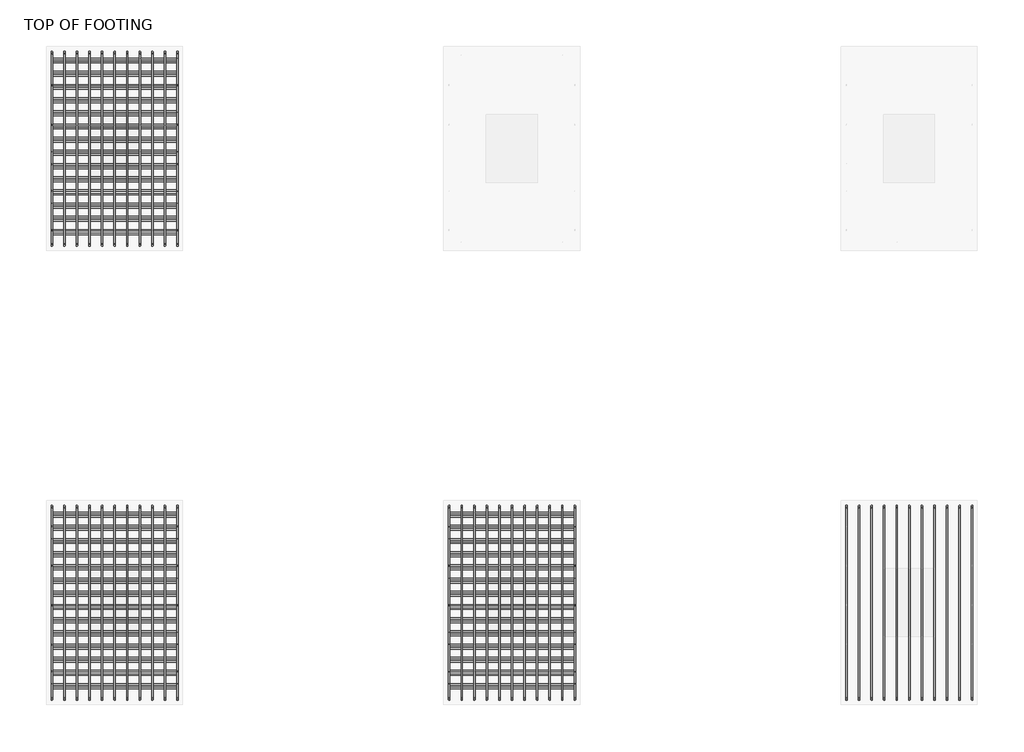
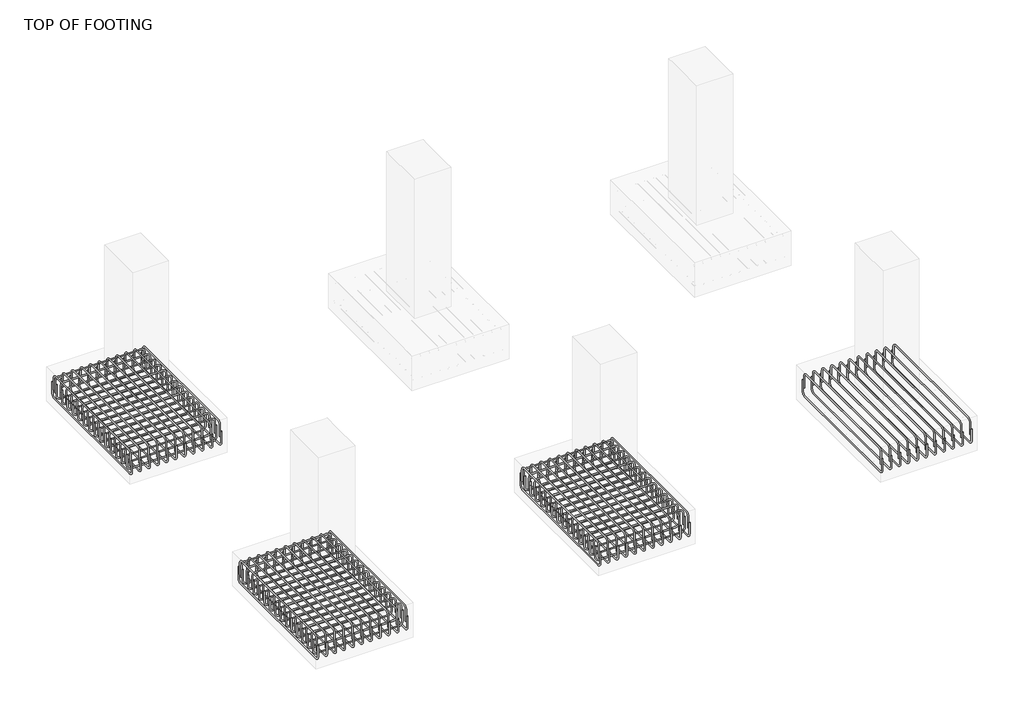
# One storey, part 3 of 11: 14 reinforcing bars.
"""IFC4 building model written with IfcOpenShell, lengths in millimetres."""

from ifc_helpers import new_model, si_unit, point, frame, origin, place, context, project, spatial, polyline, circle_curve, trimmed, segment, composite_curve, source, transform, mapped, element, save
from ifc_brep_helpers import swept_disk

model = new_model("IFC4")

# Units and contexts
model_context = context("Model", 3, world=origin())
ifc_project = project(units=[si_unit("LENGTHUNIT", "METRE", prefix="MILLI")], contexts=[model_context])

# Site, building, storey
site = spatial("IfcSite", under=ifc_project)
building = spatial("IfcBuilding", under=site)
storey = spatial("IfcBuildingStorey", under=building, Name="TOP OF FOOTING", Elevation=-1828.8)

# Reinforcing bars
placement = place(None, origin())
reinforcing_bar_shape = source(origin(), model_context, "Body", "SolidModel", [
    swept_disk(composite_curve([segment(polyline([(-8816.2384094, 6549.4712443, -2012.1658531), (-8816.2384094, 6549.4712443, -2159.4658531)]), True, "CONTINUOUS"), segment(trimmed(circle_curve(frame((-8816.2384094, 6595.8212443, -2159.4658531), z_axis=(1.0, 0.0, 0.0), x_axis=(0.0, -46.350000000000364, 0.0)), 46.35), [point((-8816.2384094, 6549.4712443, -2159.4658531))], [point((-8816.2384094, 6595.8212443, -2205.8158531))], True, "CARTESIAN"), True, "CONTINUOUS"), segment(polyline([(-8816.2384094, 6595.8212443, -2205.8158531), (-8816.2384094, 8210.4212443, -2205.8158531)]), True, "CONTINUOUS"), segment(trimmed(circle_curve(frame((-8816.2384094, 8210.4212443, -2159.4658531), z_axis=(1.0, 0.0, 0.0), x_axis=(0.0, 0.0, -46.34999999999991)), 46.35), [point((-8816.2384094, 8210.4212443, -2205.8158531))], [point((-8816.2384094, 8256.7712443, -2159.4658531))], True, "CARTESIAN"), True, "CONTINUOUS"), segment(polyline([(-8816.2384094, 8256.7712443, -2159.4658531), (-8816.2384094, 8256.7712443, -2012.1658531)]), True, "CONTINUOUS")], self_intersect=False), 6.35),
])
element("IfcReinforcingBar", 1, at=placement, inside=storey, context=model_context, shape_type="MappedRepresentation", body=[
    mapped(reinforcing_bar_shape, transform((0.0, 0.0, 0.0), x_axis=(1.0, 0.0, 0.0), y_axis=(0.0, 1.0, 0.0), z_axis=(0.0, 0.0, 1.0))),
    mapped(reinforcing_bar_shape, transform((-110.73, 0.0, 0.0), x_axis=(1.0, 0.0, 0.0), y_axis=(0.0, 1.0, 0.0), z_axis=(0.0, 0.0, 1.0))),
    mapped(reinforcing_bar_shape, transform((-221.46, 0.0, 0.0), x_axis=(1.0, 0.0, 0.0), y_axis=(0.0, 1.0, 0.0), z_axis=(0.0, 0.0, 1.0))),
    mapped(reinforcing_bar_shape, transform((-332.19, 0.0, 0.0), x_axis=(1.0, 0.0, 0.0), y_axis=(0.0, 1.0, 0.0), z_axis=(0.0, 0.0, 1.0))),
    mapped(reinforcing_bar_shape, transform((-442.92, 0.0, 0.0), x_axis=(1.0, 0.0, 0.0), y_axis=(0.0, 1.0, 0.0), z_axis=(0.0, 0.0, 1.0))),
    mapped(reinforcing_bar_shape, transform((-553.65, 0.0, 0.0), x_axis=(1.0, 0.0, 0.0), y_axis=(0.0, 1.0, 0.0), z_axis=(0.0, 0.0, 1.0))),
    mapped(reinforcing_bar_shape, transform((-664.38, 0.0, 0.0), x_axis=(1.0, 0.0, 0.0), y_axis=(0.0, 1.0, 0.0), z_axis=(0.0, 0.0, 1.0))),
    mapped(reinforcing_bar_shape, transform((-775.11, 0.0, 0.0), x_axis=(1.0, 0.0, 0.0), y_axis=(0.0, 1.0, 0.0), z_axis=(0.0, 0.0, 1.0))),
    mapped(reinforcing_bar_shape, transform((-885.84, 0.0, 0.0), x_axis=(1.0, 0.0, 0.0), y_axis=(0.0, 1.0, 0.0), z_axis=(0.0, 0.0, 1.0))),
    mapped(reinforcing_bar_shape, transform((-996.57, 0.0, 0.0), x_axis=(1.0, 0.0, 0.0), y_axis=(0.0, 1.0, 0.0), z_axis=(0.0, 0.0, 1.0))),
    mapped(reinforcing_bar_shape, transform((-1107.3, 0.0, 0.0), x_axis=(1.0, 0.0, 0.0), y_axis=(0.0, 1.0, 0.0), z_axis=(0.0, 0.0, 1.0))),
])
reinforcing_bar_2_shape = source(origin(), model_context, "Body", "SolidModel", [
    swept_disk(composite_curve([segment(polyline([(-9923.5384094, 6577.6603603, -2096.8914539), (-9923.5384094, 6577.6603603, -1949.5914539)]), True, "CONTINUOUS"), segment(trimmed(circle_curve(frame((-9923.5384094, 6624.0103603, -1949.5914539), z_axis=(-1.0, 0.0, 0.0), x_axis=(0.0, -46.349999999999454, 0.0)), 46.35), [point((-9923.5384094, 6577.6603603, -1949.5914539))], [point((-9923.5384094, 6624.0103603, -1903.2414539))], True, "CARTESIAN"), True, "CONTINUOUS"), segment(polyline([(-9923.5384094, 6624.0103603, -1903.2414539), (-9923.5384094, 8181.3238837, -1903.2414539)]), True, "CONTINUOUS"), segment(trimmed(circle_curve(frame((-9923.5384094, 8181.3238837, -1949.5914539), z_axis=(-1.0, 0.0, 0.0), x_axis=(0.0, 0.0, 46.350000000000136)), 46.35), [point((-9923.5384094, 8181.3238837, -1903.2414539))], [point((-9923.5384094, 8227.6738837, -1949.5914539))], True, "CARTESIAN"), True, "CONTINUOUS"), segment(polyline([(-9923.5384094, 8227.6738837, -1949.5914539), (-9923.5384094, 8227.6738837, -2096.8914539)]), True, "CONTINUOUS")], self_intersect=False), 6.35),
])
element("IfcReinforcingBar", 2, at=placement, inside=storey, context=model_context, shape_type="MappedRepresentation", body=[
    mapped(reinforcing_bar_2_shape, transform((0.0, 0.0, 0.0), x_axis=(1.0, 0.0, 0.0), y_axis=(0.0, 1.0, 0.0), z_axis=(0.0, 0.0, 1.0))),
    mapped(reinforcing_bar_2_shape, transform((110.73, 0.0, 0.0), x_axis=(1.0, 0.0, 0.0), y_axis=(0.0, 1.0, 0.0), z_axis=(0.0, 0.0, 1.0))),
    mapped(reinforcing_bar_2_shape, transform((221.46, 0.0, 0.0), x_axis=(1.0, 0.0, 0.0), y_axis=(0.0, 1.0, 0.0), z_axis=(0.0, 0.0, 1.0))),
    mapped(reinforcing_bar_2_shape, transform((332.19, 0.0, 0.0), x_axis=(1.0, 0.0, 0.0), y_axis=(0.0, 1.0, 0.0), z_axis=(0.0, 0.0, 1.0))),
    mapped(reinforcing_bar_2_shape, transform((442.92, 0.0, 0.0), x_axis=(1.0, 0.0, 0.0), y_axis=(0.0, 1.0, 0.0), z_axis=(0.0, 0.0, 1.0))),
    mapped(reinforcing_bar_2_shape, transform((553.65, 0.0, 0.0), x_axis=(1.0, 0.0, 0.0), y_axis=(0.0, 1.0, 0.0), z_axis=(0.0, 0.0, 1.0))),
    mapped(reinforcing_bar_2_shape, transform((664.38, 0.0, 0.0), x_axis=(1.0, 0.0, 0.0), y_axis=(0.0, 1.0, 0.0), z_axis=(0.0, 0.0, 1.0))),
    mapped(reinforcing_bar_2_shape, transform((775.11, 0.0, 0.0), x_axis=(1.0, 0.0, 0.0), y_axis=(0.0, 1.0, 0.0), z_axis=(0.0, 0.0, 1.0))),
    mapped(reinforcing_bar_2_shape, transform((885.84, 0.0, 0.0), x_axis=(1.0, 0.0, 0.0), y_axis=(0.0, 1.0, 0.0), z_axis=(0.0, 0.0, 1.0))),
    mapped(reinforcing_bar_2_shape, transform((996.57, 0.0, 0.0), x_axis=(1.0, 0.0, 0.0), y_axis=(0.0, 1.0, 0.0), z_axis=(0.0, 0.0, 1.0))),
    mapped(reinforcing_bar_2_shape, transform((1107.3, 0.0, 0.0), x_axis=(1.0, 0.0, 0.0), y_axis=(0.0, 1.0, 0.0), z_axis=(0.0, 0.0, 1.0))),
])
reinforcing_bar_3_shape = source(origin(), model_context, "Body", "SolidModel", [
    swept_disk(composite_curve([segment(polyline([(-9923.5384094, 6653.1930221, -1996.7664426), (-9923.5384094, 6653.1930221, -2144.0664426)]), True, "CONTINUOUS"), segment(trimmed(circle_curve(frame((-9877.1884094, 6653.1930221, -2144.0664426), z_axis=(0.0, -1.0, 0.0), x_axis=(-46.350000000000364, 0.0, 0.0)), 46.35), [point((-9923.5384094, 6653.1930221, -2144.0664426))], [point((-9877.1884094, 6653.1930221, -2190.4164426))], True, "CARTESIAN"), True, "CONTINUOUS"), segment(polyline([(-9877.1884094, 6653.1930221, -2190.4164426), (-8862.5884094, 6653.1930221, -2190.4164426)]), True, "CONTINUOUS"), segment(trimmed(circle_curve(frame((-8862.5884094, 6653.1930221, -2144.0664426), z_axis=(0.0, -1.0, 0.0), x_axis=(0.0, 0.0, -46.350000000000364)), 46.35), [point((-8862.5884094, 6653.1930221, -2190.4164426))], [point((-8816.2384094, 6653.1930221, -2144.0664426))], True, "CARTESIAN"), True, "CONTINUOUS"), segment(polyline([(-8816.2384094, 6653.1930221, -2144.0664426), (-8816.2384094, 6653.1930221, -1996.7664426)]), True, "CONTINUOUS")], self_intersect=False), 6.35),
])
element("IfcReinforcingBar", 3, at=placement, inside=storey, context=model_context, shape_type="MappedRepresentation", body=[
    mapped(reinforcing_bar_3_shape, transform((0.0, 0.0, 0.0), x_axis=(1.0, 0.0, 0.0), y_axis=(0.0, 1.0, 0.0), z_axis=(0.0, 0.0, 1.0))),
    mapped(reinforcing_bar_3_shape, transform((0.0, 116.2744005, 0.0), x_axis=(1.0, 0.0, 0.0), y_axis=(0.0, 1.0, 0.0), z_axis=(0.0, 0.0, 1.0))),
    mapped(reinforcing_bar_3_shape, transform((0.0, 232.5488009, 0.0), x_axis=(1.0, 0.0, 0.0), y_axis=(0.0, 1.0, 0.0), z_axis=(0.0, 0.0, 1.0))),
    mapped(reinforcing_bar_3_shape, transform((0.0, 348.8232014, 0.0), x_axis=(1.0, 0.0, 0.0), y_axis=(0.0, 1.0, 0.0), z_axis=(0.0, 0.0, 1.0))),
    mapped(reinforcing_bar_3_shape, transform((0.0, 465.0976018, 0.0), x_axis=(1.0, 0.0, 0.0), y_axis=(0.0, 1.0, 0.0), z_axis=(0.0, 0.0, 1.0))),
    mapped(reinforcing_bar_3_shape, transform((0.0, 581.3720023, 0.0), x_axis=(1.0, 0.0, 0.0), y_axis=(0.0, 1.0, 0.0), z_axis=(0.0, 0.0, 1.0))),
    mapped(reinforcing_bar_3_shape, transform((0.0, 697.6464027, 0.0), x_axis=(1.0, 0.0, 0.0), y_axis=(0.0, 1.0, 0.0), z_axis=(0.0, 0.0, 1.0))),
    mapped(reinforcing_bar_3_shape, transform((0.0, 813.9208032, 0.0), x_axis=(1.0, 0.0, 0.0), y_axis=(0.0, 1.0, 0.0), z_axis=(0.0, 0.0, 1.0))),
    mapped(reinforcing_bar_3_shape, transform((0.0, 930.1952036, 0.0), x_axis=(1.0, 0.0, 0.0), y_axis=(0.0, 1.0, 0.0), z_axis=(0.0, 0.0, 1.0))),
    mapped(reinforcing_bar_3_shape, transform((0.0, 1046.4696041, 0.0), x_axis=(1.0, 0.0, 0.0), y_axis=(0.0, 1.0, 0.0), z_axis=(0.0, 0.0, 1.0))),
    mapped(reinforcing_bar_3_shape, transform((0.0, 1162.7440045, 0.0), x_axis=(1.0, 0.0, 0.0), y_axis=(0.0, 1.0, 0.0), z_axis=(0.0, 0.0, 1.0))),
    mapped(reinforcing_bar_3_shape, transform((0.0, 1279.018405, 0.0), x_axis=(1.0, 0.0, 0.0), y_axis=(0.0, 1.0, 0.0), z_axis=(0.0, 0.0, 1.0))),
    mapped(reinforcing_bar_3_shape, transform((0.0, 1395.2928054, 0.0), x_axis=(1.0, 0.0, 0.0), y_axis=(0.0, 1.0, 0.0), z_axis=(0.0, 0.0, 1.0))),
    mapped(reinforcing_bar_3_shape, transform((0.0, 1511.5672059, 0.0), x_axis=(1.0, 0.0, 0.0), y_axis=(0.0, 1.0, 0.0), z_axis=(0.0, 0.0, 1.0))),
])
reinforcing_bar_4_shape = source(origin(), model_context, "Body", "SolidModel", [
    swept_disk(composite_curve([segment(polyline([(-9923.5384094, 8194.4257435, -2114.1958609), (-9923.5384094, 8194.4257435, -1966.8958609)]), True, "CONTINUOUS"), segment(trimmed(circle_curve(frame((-9877.1884094, 8194.4257435, -1966.8958609), z_axis=(0.0, 1.0, 0.0), x_axis=(-46.350000000000364, 0.0, 0.0)), 46.35), [point((-9923.5384094, 8194.4257435, -1966.8958609))], [point((-9877.1884094, 8194.4257435, -1920.5458609))], True, "CARTESIAN"), True, "CONTINUOUS"), segment(polyline([(-9877.1884094, 8194.4257435, -1920.5458609), (-8862.5884094, 8194.4257435, -1920.5458609)]), True, "CONTINUOUS"), segment(trimmed(circle_curve(frame((-8862.5884094, 8194.4257435, -1966.8958609), z_axis=(0.0, 1.0, 0.0), x_axis=(0.0, 0.0, 46.34999999999991)), 46.35), [point((-8862.5884094, 8194.4257435, -1920.5458609))], [point((-8816.2384094, 8194.4257435, -1966.8958609))], True, "CARTESIAN"), True, "CONTINUOUS"), segment(polyline([(-8816.2384094, 8194.4257435, -1966.8958609), (-8816.2384094, 8194.4257435, -2114.1958609)]), True, "CONTINUOUS")], self_intersect=False), 6.35),
])
element("IfcReinforcingBar", 4, at=placement, inside=storey, context=model_context, shape_type="MappedRepresentation", body=[
    mapped(reinforcing_bar_4_shape, transform((0.0, 0.0, 0.0), x_axis=(1.0, 0.0, 0.0), y_axis=(0.0, 1.0, 0.0), z_axis=(0.0, 0.0, 1.0))),
    mapped(reinforcing_bar_4_shape, transform((0.0, -116.1057918, 0.0), x_axis=(1.0, 0.0, 0.0), y_axis=(0.0, 1.0, 0.0), z_axis=(0.0, 0.0, 1.0))),
    mapped(reinforcing_bar_4_shape, transform((0.0, -232.2115836, 0.0), x_axis=(1.0, 0.0, 0.0), y_axis=(0.0, 1.0, 0.0), z_axis=(0.0, 0.0, 1.0))),
    mapped(reinforcing_bar_4_shape, transform((0.0, -348.3173754, 0.0), x_axis=(1.0, 0.0, 0.0), y_axis=(0.0, 1.0, 0.0), z_axis=(0.0, 0.0, 1.0))),
    mapped(reinforcing_bar_4_shape, transform((0.0, -464.4231672, 0.0), x_axis=(1.0, 0.0, 0.0), y_axis=(0.0, 1.0, 0.0), z_axis=(0.0, 0.0, 1.0))),
    mapped(reinforcing_bar_4_shape, transform((0.0, -580.528959, 0.0), x_axis=(1.0, 0.0, 0.0), y_axis=(0.0, 1.0, 0.0), z_axis=(0.0, 0.0, 1.0))),
    mapped(reinforcing_bar_4_shape, transform((0.0, -696.6347508, 0.0), x_axis=(1.0, 0.0, 0.0), y_axis=(0.0, 1.0, 0.0), z_axis=(0.0, 0.0, 1.0))),
    mapped(reinforcing_bar_4_shape, transform((0.0, -812.7405426, 0.0), x_axis=(1.0, 0.0, 0.0), y_axis=(0.0, 1.0, 0.0), z_axis=(0.0, 0.0, 1.0))),
    mapped(reinforcing_bar_4_shape, transform((0.0, -928.8463344, 0.0), x_axis=(1.0, 0.0, 0.0), y_axis=(0.0, 1.0, 0.0), z_axis=(0.0, 0.0, 1.0))),
    mapped(reinforcing_bar_4_shape, transform((0.0, -1044.9521262, 0.0), x_axis=(1.0, 0.0, 0.0), y_axis=(0.0, 1.0, 0.0), z_axis=(0.0, 0.0, 1.0))),
    mapped(reinforcing_bar_4_shape, transform((0.0, -1161.057918, 0.0), x_axis=(1.0, 0.0, 0.0), y_axis=(0.0, 1.0, 0.0), z_axis=(0.0, 0.0, 1.0))),
    mapped(reinforcing_bar_4_shape, transform((0.0, -1277.1637098, 0.0), x_axis=(1.0, 0.0, 0.0), y_axis=(0.0, 1.0, 0.0), z_axis=(0.0, 0.0, 1.0))),
    mapped(reinforcing_bar_4_shape, transform((0.0, -1393.2695016, 0.0), x_axis=(1.0, 0.0, 0.0), y_axis=(0.0, 1.0, 0.0), z_axis=(0.0, 0.0, 1.0))),
    mapped(reinforcing_bar_4_shape, transform((0.0, -1509.3752934, 0.0), x_axis=(1.0, 0.0, 0.0), y_axis=(0.0, 1.0, 0.0), z_axis=(0.0, 0.0, 1.0))),
])
reinforcing_bar_5_shape = source(origin(), model_context, "Body", "SolidModel", [
    swept_disk(composite_curve([segment(polyline([(-8816.2384094, 2549.4712443, -2012.1658531), (-8816.2384094, 2549.4712443, -2159.4658531)]), True, "CONTINUOUS"), segment(trimmed(circle_curve(frame((-8816.2384094, 2595.8212443, -2159.4658531), z_axis=(1.0, 0.0, 0.0), x_axis=(0.0, -46.350000000000364, 0.0)), 46.35), [point((-8816.2384094, 2549.4712443, -2159.4658531))], [point((-8816.2384094, 2595.8212443, -2205.8158531))], True, "CARTESIAN"), True, "CONTINUOUS"), segment(polyline([(-8816.2384094, 2595.8212443, -2205.8158531), (-8816.2384094, 4210.4212443, -2205.8158531)]), True, "CONTINUOUS"), segment(trimmed(circle_curve(frame((-8816.2384094, 4210.4212443, -2159.4658531), z_axis=(1.0, 0.0, 0.0), x_axis=(0.0, 0.0, -46.34999999999991)), 46.35), [point((-8816.2384094, 4210.4212443, -2205.8158531))], [point((-8816.2384094, 4256.7712443, -2159.4658531))], True, "CARTESIAN"), True, "CONTINUOUS"), segment(polyline([(-8816.2384094, 4256.7712443, -2159.4658531), (-8816.2384094, 4256.7712443, -2012.1658531)]), True, "CONTINUOUS")], self_intersect=False), 6.35),
])
element("IfcReinforcingBar", 5, at=placement, inside=storey, context=model_context, shape_type="MappedRepresentation", body=[
    mapped(reinforcing_bar_5_shape, transform((0.0, 0.0, 0.0), x_axis=(1.0, 0.0, 0.0), y_axis=(0.0, 1.0, 0.0), z_axis=(0.0, 0.0, 1.0))),
    mapped(reinforcing_bar_5_shape, transform((-110.73, 0.0, 0.0), x_axis=(1.0, 0.0, 0.0), y_axis=(0.0, 1.0, 0.0), z_axis=(0.0, 0.0, 1.0))),
    mapped(reinforcing_bar_5_shape, transform((-221.46, 0.0, 0.0), x_axis=(1.0, 0.0, 0.0), y_axis=(0.0, 1.0, 0.0), z_axis=(0.0, 0.0, 1.0))),
    mapped(reinforcing_bar_5_shape, transform((-332.19, 0.0, 0.0), x_axis=(1.0, 0.0, 0.0), y_axis=(0.0, 1.0, 0.0), z_axis=(0.0, 0.0, 1.0))),
    mapped(reinforcing_bar_5_shape, transform((-442.92, 0.0, 0.0), x_axis=(1.0, 0.0, 0.0), y_axis=(0.0, 1.0, 0.0), z_axis=(0.0, 0.0, 1.0))),
    mapped(reinforcing_bar_5_shape, transform((-553.65, 0.0, 0.0), x_axis=(1.0, 0.0, 0.0), y_axis=(0.0, 1.0, 0.0), z_axis=(0.0, 0.0, 1.0))),
    mapped(reinforcing_bar_5_shape, transform((-664.38, 0.0, 0.0), x_axis=(1.0, 0.0, 0.0), y_axis=(0.0, 1.0, 0.0), z_axis=(0.0, 0.0, 1.0))),
    mapped(reinforcing_bar_5_shape, transform((-775.11, 0.0, 0.0), x_axis=(1.0, 0.0, 0.0), y_axis=(0.0, 1.0, 0.0), z_axis=(0.0, 0.0, 1.0))),
    mapped(reinforcing_bar_5_shape, transform((-885.84, 0.0, 0.0), x_axis=(1.0, 0.0, 0.0), y_axis=(0.0, 1.0, 0.0), z_axis=(0.0, 0.0, 1.0))),
    mapped(reinforcing_bar_5_shape, transform((-996.57, 0.0, 0.0), x_axis=(1.0, 0.0, 0.0), y_axis=(0.0, 1.0, 0.0), z_axis=(0.0, 0.0, 1.0))),
    mapped(reinforcing_bar_5_shape, transform((-1107.3, 0.0, 0.0), x_axis=(1.0, 0.0, 0.0), y_axis=(0.0, 1.0, 0.0), z_axis=(0.0, 0.0, 1.0))),
])
reinforcing_bar_6_shape = source(origin(), model_context, "Body", "SolidModel", [
    swept_disk(composite_curve([segment(polyline([(-9923.5384094, 2577.6603603, -2096.8914539), (-9923.5384094, 2577.6603603, -1949.5914539)]), True, "CONTINUOUS"), segment(trimmed(circle_curve(frame((-9923.5384094, 2624.0103603, -1949.5914539), z_axis=(-1.0, 0.0, 0.0), x_axis=(0.0, -46.34999999999991, 0.0)), 46.35), [point((-9923.5384094, 2577.6603603, -1949.5914539))], [point((-9923.5384094, 2624.0103603, -1903.2414539))], True, "CARTESIAN"), True, "CONTINUOUS"), segment(polyline([(-9923.5384094, 2624.0103603, -1903.2414539), (-9923.5384094, 4181.3238837, -1903.2414539)]), True, "CONTINUOUS"), segment(trimmed(circle_curve(frame((-9923.5384094, 4181.3238837, -1949.5914539), z_axis=(-1.0, 0.0, 0.0), x_axis=(0.0, 0.0, 46.350000000000136)), 46.35), [point((-9923.5384094, 4181.3238837, -1903.2414539))], [point((-9923.5384094, 4227.6738837, -1949.5914539))], True, "CARTESIAN"), True, "CONTINUOUS"), segment(polyline([(-9923.5384094, 4227.6738837, -1949.5914539), (-9923.5384094, 4227.6738837, -2096.8914539)]), True, "CONTINUOUS")], self_intersect=False), 6.35),
])
element("IfcReinforcingBar", 6, at=placement, inside=storey, context=model_context, shape_type="MappedRepresentation", body=[
    mapped(reinforcing_bar_6_shape, transform((0.0, 0.0, 0.0), x_axis=(1.0, 0.0, 0.0), y_axis=(0.0, 1.0, 0.0), z_axis=(0.0, 0.0, 1.0))),
    mapped(reinforcing_bar_6_shape, transform((110.73, 0.0, 0.0), x_axis=(1.0, 0.0, 0.0), y_axis=(0.0, 1.0, 0.0), z_axis=(0.0, 0.0, 1.0))),
    mapped(reinforcing_bar_6_shape, transform((221.46, 0.0, 0.0), x_axis=(1.0, 0.0, 0.0), y_axis=(0.0, 1.0, 0.0), z_axis=(0.0, 0.0, 1.0))),
    mapped(reinforcing_bar_6_shape, transform((332.19, 0.0, 0.0), x_axis=(1.0, 0.0, 0.0), y_axis=(0.0, 1.0, 0.0), z_axis=(0.0, 0.0, 1.0))),
    mapped(reinforcing_bar_6_shape, transform((442.92, 0.0, 0.0), x_axis=(1.0, 0.0, 0.0), y_axis=(0.0, 1.0, 0.0), z_axis=(0.0, 0.0, 1.0))),
    mapped(reinforcing_bar_6_shape, transform((553.65, 0.0, 0.0), x_axis=(1.0, 0.0, 0.0), y_axis=(0.0, 1.0, 0.0), z_axis=(0.0, 0.0, 1.0))),
    mapped(reinforcing_bar_6_shape, transform((664.38, 0.0, 0.0), x_axis=(1.0, 0.0, 0.0), y_axis=(0.0, 1.0, 0.0), z_axis=(0.0, 0.0, 1.0))),
    mapped(reinforcing_bar_6_shape, transform((775.11, 0.0, 0.0), x_axis=(1.0, 0.0, 0.0), y_axis=(0.0, 1.0, 0.0), z_axis=(0.0, 0.0, 1.0))),
    mapped(reinforcing_bar_6_shape, transform((885.84, 0.0, 0.0), x_axis=(1.0, 0.0, 0.0), y_axis=(0.0, 1.0, 0.0), z_axis=(0.0, 0.0, 1.0))),
    mapped(reinforcing_bar_6_shape, transform((996.57, 0.0, 0.0), x_axis=(1.0, 0.0, 0.0), y_axis=(0.0, 1.0, 0.0), z_axis=(0.0, 0.0, 1.0))),
    mapped(reinforcing_bar_6_shape, transform((1107.3, 0.0, 0.0), x_axis=(1.0, 0.0, 0.0), y_axis=(0.0, 1.0, 0.0), z_axis=(0.0, 0.0, 1.0))),
])
reinforcing_bar_7_shape = source(origin(), model_context, "Body", "SolidModel", [
    swept_disk(composite_curve([segment(polyline([(-9923.5384094, 2653.1930221, -1996.7664426), (-9923.5384094, 2653.1930221, -2144.0664426)]), True, "CONTINUOUS"), segment(trimmed(circle_curve(frame((-9877.1884094, 2653.1930221, -2144.0664426), z_axis=(0.0, -1.0, 0.0), x_axis=(-46.350000000000364, 0.0, 0.0)), 46.35), [point((-9923.5384094, 2653.1930221, -2144.0664426))], [point((-9877.1884094, 2653.1930221, -2190.4164426))], True, "CARTESIAN"), True, "CONTINUOUS"), segment(polyline([(-9877.1884094, 2653.1930221, -2190.4164426), (-8862.5884094, 2653.1930221, -2190.4164426)]), True, "CONTINUOUS"), segment(trimmed(circle_curve(frame((-8862.5884094, 2653.1930221, -2144.0664426), z_axis=(0.0, -1.0, 0.0), x_axis=(0.0, 0.0, -46.350000000000364)), 46.35), [point((-8862.5884094, 2653.1930221, -2190.4164426))], [point((-8816.2384094, 2653.1930221, -2144.0664426))], True, "CARTESIAN"), True, "CONTINUOUS"), segment(polyline([(-8816.2384094, 2653.1930221, -2144.0664426), (-8816.2384094, 2653.1930221, -1996.7664426)]), True, "CONTINUOUS")], self_intersect=False), 6.35),
])
element("IfcReinforcingBar", 7, at=placement, inside=storey, context=model_context, shape_type="MappedRepresentation", body=[
    mapped(reinforcing_bar_7_shape, transform((0.0, 0.0, 0.0), x_axis=(1.0, 0.0, 0.0), y_axis=(0.0, 1.0, 0.0), z_axis=(0.0, 0.0, 1.0))),
    mapped(reinforcing_bar_7_shape, transform((0.0, 116.2744005, 0.0), x_axis=(1.0, 0.0, 0.0), y_axis=(0.0, 1.0, 0.0), z_axis=(0.0, 0.0, 1.0))),
    mapped(reinforcing_bar_7_shape, transform((0.0, 232.5488009, 0.0), x_axis=(1.0, 0.0, 0.0), y_axis=(0.0, 1.0, 0.0), z_axis=(0.0, 0.0, 1.0))),
    mapped(reinforcing_bar_7_shape, transform((0.0, 348.8232014, 0.0), x_axis=(1.0, 0.0, 0.0), y_axis=(0.0, 1.0, 0.0), z_axis=(0.0, 0.0, 1.0))),
    mapped(reinforcing_bar_7_shape, transform((0.0, 465.0976018, 0.0), x_axis=(1.0, 0.0, 0.0), y_axis=(0.0, 1.0, 0.0), z_axis=(0.0, 0.0, 1.0))),
    mapped(reinforcing_bar_7_shape, transform((0.0, 581.3720023, 0.0), x_axis=(1.0, 0.0, 0.0), y_axis=(0.0, 1.0, 0.0), z_axis=(0.0, 0.0, 1.0))),
    mapped(reinforcing_bar_7_shape, transform((0.0, 697.6464027, 0.0), x_axis=(1.0, 0.0, 0.0), y_axis=(0.0, 1.0, 0.0), z_axis=(0.0, 0.0, 1.0))),
    mapped(reinforcing_bar_7_shape, transform((0.0, 813.9208032, 0.0), x_axis=(1.0, 0.0, 0.0), y_axis=(0.0, 1.0, 0.0), z_axis=(0.0, 0.0, 1.0))),
    mapped(reinforcing_bar_7_shape, transform((0.0, 930.1952036, 0.0), x_axis=(1.0, 0.0, 0.0), y_axis=(0.0, 1.0, 0.0), z_axis=(0.0, 0.0, 1.0))),
    mapped(reinforcing_bar_7_shape, transform((0.0, 1046.4696041, 0.0), x_axis=(1.0, 0.0, 0.0), y_axis=(0.0, 1.0, 0.0), z_axis=(0.0, 0.0, 1.0))),
    mapped(reinforcing_bar_7_shape, transform((0.0, 1162.7440045, 0.0), x_axis=(1.0, 0.0, 0.0), y_axis=(0.0, 1.0, 0.0), z_axis=(0.0, 0.0, 1.0))),
    mapped(reinforcing_bar_7_shape, transform((0.0, 1279.018405, 0.0), x_axis=(1.0, 0.0, 0.0), y_axis=(0.0, 1.0, 0.0), z_axis=(0.0, 0.0, 1.0))),
    mapped(reinforcing_bar_7_shape, transform((0.0, 1395.2928054, 0.0), x_axis=(1.0, 0.0, 0.0), y_axis=(0.0, 1.0, 0.0), z_axis=(0.0, 0.0, 1.0))),
    mapped(reinforcing_bar_7_shape, transform((0.0, 1511.5672059, 0.0), x_axis=(1.0, 0.0, 0.0), y_axis=(0.0, 1.0, 0.0), z_axis=(0.0, 0.0, 1.0))),
])
reinforcing_bar_8_shape = source(origin(), model_context, "Body", "SolidModel", [
    swept_disk(composite_curve([segment(polyline([(-9923.5384094, 4194.4257435, -2114.1958609), (-9923.5384094, 4194.4257435, -1966.8958609)]), True, "CONTINUOUS"), segment(trimmed(circle_curve(frame((-9877.1884094, 4194.4257435, -1966.8958609), z_axis=(0.0, 1.0, 0.0), x_axis=(-46.350000000000364, 0.0, 0.0)), 46.35), [point((-9923.5384094, 4194.4257435, -1966.8958609))], [point((-9877.1884094, 4194.4257435, -1920.5458609))], True, "CARTESIAN"), True, "CONTINUOUS"), segment(polyline([(-9877.1884094, 4194.4257435, -1920.5458609), (-8862.5884094, 4194.4257435, -1920.5458609)]), True, "CONTINUOUS"), segment(trimmed(circle_curve(frame((-8862.5884094, 4194.4257435, -1966.8958609), z_axis=(0.0, 1.0, 0.0), x_axis=(0.0, 0.0, 46.34999999999991)), 46.35), [point((-8862.5884094, 4194.4257435, -1920.5458609))], [point((-8816.2384094, 4194.4257435, -1966.8958609))], True, "CARTESIAN"), True, "CONTINUOUS"), segment(polyline([(-8816.2384094, 4194.4257435, -1966.8958609), (-8816.2384094, 4194.4257435, -2114.1958609)]), True, "CONTINUOUS")], self_intersect=False), 6.35),
])
element("IfcReinforcingBar", 8, at=placement, inside=storey, context=model_context, shape_type="MappedRepresentation", body=[
    mapped(reinforcing_bar_8_shape, transform((0.0, 0.0, 0.0), x_axis=(1.0, 0.0, 0.0), y_axis=(0.0, 1.0, 0.0), z_axis=(0.0, 0.0, 1.0))),
    mapped(reinforcing_bar_8_shape, transform((0.0, -116.1057918, 0.0), x_axis=(1.0, 0.0, 0.0), y_axis=(0.0, 1.0, 0.0), z_axis=(0.0, 0.0, 1.0))),
    mapped(reinforcing_bar_8_shape, transform((0.0, -232.2115836, 0.0), x_axis=(1.0, 0.0, 0.0), y_axis=(0.0, 1.0, 0.0), z_axis=(0.0, 0.0, 1.0))),
    mapped(reinforcing_bar_8_shape, transform((0.0, -348.3173754, 0.0), x_axis=(1.0, 0.0, 0.0), y_axis=(0.0, 1.0, 0.0), z_axis=(0.0, 0.0, 1.0))),
    mapped(reinforcing_bar_8_shape, transform((0.0, -464.4231672, 0.0), x_axis=(1.0, 0.0, 0.0), y_axis=(0.0, 1.0, 0.0), z_axis=(0.0, 0.0, 1.0))),
    mapped(reinforcing_bar_8_shape, transform((0.0, -580.528959, 0.0), x_axis=(1.0, 0.0, 0.0), y_axis=(0.0, 1.0, 0.0), z_axis=(0.0, 0.0, 1.0))),
    mapped(reinforcing_bar_8_shape, transform((0.0, -696.6347508, 0.0), x_axis=(1.0, 0.0, 0.0), y_axis=(0.0, 1.0, 0.0), z_axis=(0.0, 0.0, 1.0))),
    mapped(reinforcing_bar_8_shape, transform((0.0, -812.7405426, 0.0), x_axis=(1.0, 0.0, 0.0), y_axis=(0.0, 1.0, 0.0), z_axis=(0.0, 0.0, 1.0))),
    mapped(reinforcing_bar_8_shape, transform((0.0, -928.8463344, 0.0), x_axis=(1.0, 0.0, 0.0), y_axis=(0.0, 1.0, 0.0), z_axis=(0.0, 0.0, 1.0))),
    mapped(reinforcing_bar_8_shape, transform((0.0, -1044.9521262, 0.0), x_axis=(1.0, 0.0, 0.0), y_axis=(0.0, 1.0, 0.0), z_axis=(0.0, 0.0, 1.0))),
    mapped(reinforcing_bar_8_shape, transform((0.0, -1161.057918, 0.0), x_axis=(1.0, 0.0, 0.0), y_axis=(0.0, 1.0, 0.0), z_axis=(0.0, 0.0, 1.0))),
    mapped(reinforcing_bar_8_shape, transform((0.0, -1277.1637098, 0.0), x_axis=(1.0, 0.0, 0.0), y_axis=(0.0, 1.0, 0.0), z_axis=(0.0, 0.0, 1.0))),
    mapped(reinforcing_bar_8_shape, transform((0.0, -1393.2695016, 0.0), x_axis=(1.0, 0.0, 0.0), y_axis=(0.0, 1.0, 0.0), z_axis=(0.0, 0.0, 1.0))),
    mapped(reinforcing_bar_8_shape, transform((0.0, -1509.3752934, 0.0), x_axis=(1.0, 0.0, 0.0), y_axis=(0.0, 1.0, 0.0), z_axis=(0.0, 0.0, 1.0))),
])
reinforcing_bar_9_shape = source(origin(), model_context, "Body", "SolidModel", [
    swept_disk(composite_curve([segment(polyline([(-1816.2384094, 2549.4712443, -2012.1658531), (-1816.2384094, 2549.4712443, -2159.4658531)]), True, "CONTINUOUS"), segment(trimmed(circle_curve(frame((-1816.2384094, 2595.8212443, -2159.4658531), z_axis=(1.0, 0.0, 0.0), x_axis=(0.0, -46.350000000000364, 0.0)), 46.35), [point((-1816.2384094, 2549.4712443, -2159.4658531))], [point((-1816.2384094, 2595.8212443, -2205.8158531))], True, "CARTESIAN"), True, "CONTINUOUS"), segment(polyline([(-1816.2384094, 2595.8212443, -2205.8158531), (-1816.2384094, 4210.4212443, -2205.8158531)]), True, "CONTINUOUS"), segment(trimmed(circle_curve(frame((-1816.2384094, 4210.4212443, -2159.4658531), z_axis=(1.0, 0.0, 0.0), x_axis=(0.0, 0.0, -46.34999999999991)), 46.35), [point((-1816.2384094, 4210.4212443, -2205.8158531))], [point((-1816.2384094, 4256.7712443, -2159.4658531))], True, "CARTESIAN"), True, "CONTINUOUS"), segment(polyline([(-1816.2384094, 4256.7712443, -2159.4658531), (-1816.2384094, 4256.7712443, -2012.1658531)]), True, "CONTINUOUS")], self_intersect=False), 6.35),
])
element("IfcReinforcingBar", 9, at=placement, inside=storey, context=model_context, shape_type="MappedRepresentation", body=[
    mapped(reinforcing_bar_9_shape, transform((0.0, 0.0, 0.0), x_axis=(1.0, 0.0, 0.0), y_axis=(0.0, 1.0, 0.0), z_axis=(0.0, 0.0, 1.0))),
    mapped(reinforcing_bar_9_shape, transform((-110.73, 0.0, 0.0), x_axis=(1.0, 0.0, 0.0), y_axis=(0.0, 1.0, 0.0), z_axis=(0.0, 0.0, 1.0))),
    mapped(reinforcing_bar_9_shape, transform((-221.46, 0.0, 0.0), x_axis=(1.0, 0.0, 0.0), y_axis=(0.0, 1.0, 0.0), z_axis=(0.0, 0.0, 1.0))),
    mapped(reinforcing_bar_9_shape, transform((-332.19, 0.0, 0.0), x_axis=(1.0, 0.0, 0.0), y_axis=(0.0, 1.0, 0.0), z_axis=(0.0, 0.0, 1.0))),
    mapped(reinforcing_bar_9_shape, transform((-442.92, 0.0, 0.0), x_axis=(1.0, 0.0, 0.0), y_axis=(0.0, 1.0, 0.0), z_axis=(0.0, 0.0, 1.0))),
    mapped(reinforcing_bar_9_shape, transform((-553.65, 0.0, 0.0), x_axis=(1.0, 0.0, 0.0), y_axis=(0.0, 1.0, 0.0), z_axis=(0.0, 0.0, 1.0))),
    mapped(reinforcing_bar_9_shape, transform((-664.38, 0.0, 0.0), x_axis=(1.0, 0.0, 0.0), y_axis=(0.0, 1.0, 0.0), z_axis=(0.0, 0.0, 1.0))),
    mapped(reinforcing_bar_9_shape, transform((-775.11, 0.0, 0.0), x_axis=(1.0, 0.0, 0.0), y_axis=(0.0, 1.0, 0.0), z_axis=(0.0, 0.0, 1.0))),
    mapped(reinforcing_bar_9_shape, transform((-885.84, 0.0, 0.0), x_axis=(1.0, 0.0, 0.0), y_axis=(0.0, 1.0, 0.0), z_axis=(0.0, 0.0, 1.0))),
    mapped(reinforcing_bar_9_shape, transform((-996.57, 0.0, 0.0), x_axis=(1.0, 0.0, 0.0), y_axis=(0.0, 1.0, 0.0), z_axis=(0.0, 0.0, 1.0))),
    mapped(reinforcing_bar_9_shape, transform((-1107.3, 0.0, 0.0), x_axis=(1.0, 0.0, 0.0), y_axis=(0.0, 1.0, 0.0), z_axis=(0.0, 0.0, 1.0))),
])
reinforcing_bar_10_shape = source(origin(), model_context, "Body", "SolidModel", [
    swept_disk(composite_curve([segment(polyline([(-2923.5384094, 2577.6603603, -2096.8914539), (-2923.5384094, 2577.6603603, -1949.5914539)]), True, "CONTINUOUS"), segment(trimmed(circle_curve(frame((-2923.5384094, 2624.0103603, -1949.5914539), z_axis=(-1.0, 0.0, 0.0), x_axis=(0.0, -46.34999999999991, 0.0)), 46.35), [point((-2923.5384094, 2577.6603603, -1949.5914539))], [point((-2923.5384094, 2624.0103603, -1903.2414539))], True, "CARTESIAN"), True, "CONTINUOUS"), segment(polyline([(-2923.5384094, 2624.0103603, -1903.2414539), (-2923.5384094, 4181.3238837, -1903.2414539)]), True, "CONTINUOUS"), segment(trimmed(circle_curve(frame((-2923.5384094, 4181.3238837, -1949.5914539), z_axis=(-1.0, 0.0, 0.0), x_axis=(0.0, 0.0, 46.350000000000136)), 46.35), [point((-2923.5384094, 4181.3238837, -1903.2414539))], [point((-2923.5384094, 4227.6738837, -1949.5914539))], True, "CARTESIAN"), True, "CONTINUOUS"), segment(polyline([(-2923.5384094, 4227.6738837, -1949.5914539), (-2923.5384094, 4227.6738837, -2096.8914539)]), True, "CONTINUOUS")], self_intersect=False), 6.35),
])
element("IfcReinforcingBar", 10, at=placement, inside=storey, context=model_context, shape_type="MappedRepresentation", body=[
    mapped(reinforcing_bar_10_shape, transform((0.0, 0.0, 0.0), x_axis=(1.0, 0.0, 0.0), y_axis=(0.0, 1.0, 0.0), z_axis=(0.0, 0.0, 1.0))),
    mapped(reinforcing_bar_10_shape, transform((110.73, 0.0, 0.0), x_axis=(1.0, 0.0, 0.0), y_axis=(0.0, 1.0, 0.0), z_axis=(0.0, 0.0, 1.0))),
    mapped(reinforcing_bar_10_shape, transform((221.46, 0.0, 0.0), x_axis=(1.0, 0.0, 0.0), y_axis=(0.0, 1.0, 0.0), z_axis=(0.0, 0.0, 1.0))),
    mapped(reinforcing_bar_10_shape, transform((332.19, 0.0, 0.0), x_axis=(1.0, 0.0, 0.0), y_axis=(0.0, 1.0, 0.0), z_axis=(0.0, 0.0, 1.0))),
    mapped(reinforcing_bar_10_shape, transform((442.92, 0.0, 0.0), x_axis=(1.0, 0.0, 0.0), y_axis=(0.0, 1.0, 0.0), z_axis=(0.0, 0.0, 1.0))),
    mapped(reinforcing_bar_10_shape, transform((553.65, 0.0, 0.0), x_axis=(1.0, 0.0, 0.0), y_axis=(0.0, 1.0, 0.0), z_axis=(0.0, 0.0, 1.0))),
    mapped(reinforcing_bar_10_shape, transform((664.38, 0.0, 0.0), x_axis=(1.0, 0.0, 0.0), y_axis=(0.0, 1.0, 0.0), z_axis=(0.0, 0.0, 1.0))),
    mapped(reinforcing_bar_10_shape, transform((775.11, 0.0, 0.0), x_axis=(1.0, 0.0, 0.0), y_axis=(0.0, 1.0, 0.0), z_axis=(0.0, 0.0, 1.0))),
    mapped(reinforcing_bar_10_shape, transform((885.84, 0.0, 0.0), x_axis=(1.0, 0.0, 0.0), y_axis=(0.0, 1.0, 0.0), z_axis=(0.0, 0.0, 1.0))),
    mapped(reinforcing_bar_10_shape, transform((996.57, 0.0, 0.0), x_axis=(1.0, 0.0, 0.0), y_axis=(0.0, 1.0, 0.0), z_axis=(0.0, 0.0, 1.0))),
    mapped(reinforcing_bar_10_shape, transform((1107.3, 0.0, 0.0), x_axis=(1.0, 0.0, 0.0), y_axis=(0.0, 1.0, 0.0), z_axis=(0.0, 0.0, 1.0))),
])
reinforcing_bar_11_shape = source(origin(), model_context, "Body", "SolidModel", [
    swept_disk(composite_curve([segment(polyline([(-5316.2384094, 2549.4712443, -2012.1658531), (-5316.2384094, 2549.4712443, -2159.4658531)]), True, "CONTINUOUS"), segment(trimmed(circle_curve(frame((-5316.2384094, 2595.8212443, -2159.4658531), z_axis=(1.0, 0.0, 0.0), x_axis=(0.0, -46.350000000000364, 0.0)), 46.35), [point((-5316.2384094, 2549.4712443, -2159.4658531))], [point((-5316.2384094, 2595.8212443, -2205.8158531))], True, "CARTESIAN"), True, "CONTINUOUS"), segment(polyline([(-5316.2384094, 2595.8212443, -2205.8158531), (-5316.2384094, 4210.4212443, -2205.8158531)]), True, "CONTINUOUS"), segment(trimmed(circle_curve(frame((-5316.2384094, 4210.4212443, -2159.4658531), z_axis=(1.0, 0.0, 0.0), x_axis=(0.0, 0.0, -46.34999999999991)), 46.35), [point((-5316.2384094, 4210.4212443, -2205.8158531))], [point((-5316.2384094, 4256.7712443, -2159.4658531))], True, "CARTESIAN"), True, "CONTINUOUS"), segment(polyline([(-5316.2384094, 4256.7712443, -2159.4658531), (-5316.2384094, 4256.7712443, -2012.1658531)]), True, "CONTINUOUS")], self_intersect=False), 6.35),
])
element("IfcReinforcingBar", 11, at=placement, inside=storey, context=model_context, shape_type="MappedRepresentation", body=[
    mapped(reinforcing_bar_11_shape, transform((0.0, 0.0, 0.0), x_axis=(1.0, 0.0, 0.0), y_axis=(0.0, 1.0, 0.0), z_axis=(0.0, 0.0, 1.0))),
    mapped(reinforcing_bar_11_shape, transform((-110.73, 0.0, 0.0), x_axis=(1.0, 0.0, 0.0), y_axis=(0.0, 1.0, 0.0), z_axis=(0.0, 0.0, 1.0))),
    mapped(reinforcing_bar_11_shape, transform((-221.46, 0.0, 0.0), x_axis=(1.0, 0.0, 0.0), y_axis=(0.0, 1.0, 0.0), z_axis=(0.0, 0.0, 1.0))),
    mapped(reinforcing_bar_11_shape, transform((-332.19, 0.0, 0.0), x_axis=(1.0, 0.0, 0.0), y_axis=(0.0, 1.0, 0.0), z_axis=(0.0, 0.0, 1.0))),
    mapped(reinforcing_bar_11_shape, transform((-442.92, 0.0, 0.0), x_axis=(1.0, 0.0, 0.0), y_axis=(0.0, 1.0, 0.0), z_axis=(0.0, 0.0, 1.0))),
    mapped(reinforcing_bar_11_shape, transform((-553.65, 0.0, 0.0), x_axis=(1.0, 0.0, 0.0), y_axis=(0.0, 1.0, 0.0), z_axis=(0.0, 0.0, 1.0))),
    mapped(reinforcing_bar_11_shape, transform((-664.38, 0.0, 0.0), x_axis=(1.0, 0.0, 0.0), y_axis=(0.0, 1.0, 0.0), z_axis=(0.0, 0.0, 1.0))),
    mapped(reinforcing_bar_11_shape, transform((-775.11, 0.0, 0.0), x_axis=(1.0, 0.0, 0.0), y_axis=(0.0, 1.0, 0.0), z_axis=(0.0, 0.0, 1.0))),
    mapped(reinforcing_bar_11_shape, transform((-885.84, 0.0, 0.0), x_axis=(1.0, 0.0, 0.0), y_axis=(0.0, 1.0, 0.0), z_axis=(0.0, 0.0, 1.0))),
    mapped(reinforcing_bar_11_shape, transform((-996.57, 0.0, 0.0), x_axis=(1.0, 0.0, 0.0), y_axis=(0.0, 1.0, 0.0), z_axis=(0.0, 0.0, 1.0))),
    mapped(reinforcing_bar_11_shape, transform((-1107.3, 0.0, 0.0), x_axis=(1.0, 0.0, 0.0), y_axis=(0.0, 1.0, 0.0), z_axis=(0.0, 0.0, 1.0))),
])
reinforcing_bar_12_shape = source(origin(), model_context, "Body", "SolidModel", [
    swept_disk(composite_curve([segment(polyline([(-6423.5384094, 2577.6603603, -2096.8914539), (-6423.5384094, 2577.6603603, -1949.5914539)]), True, "CONTINUOUS"), segment(trimmed(circle_curve(frame((-6423.5384094, 2624.0103603, -1949.5914539), z_axis=(-1.0, 0.0, 0.0), x_axis=(0.0, -46.34999999999991, 0.0)), 46.35), [point((-6423.5384094, 2577.6603603, -1949.5914539))], [point((-6423.5384094, 2624.0103603, -1903.2414539))], True, "CARTESIAN"), True, "CONTINUOUS"), segment(polyline([(-6423.5384094, 2624.0103603, -1903.2414539), (-6423.5384094, 4181.3238837, -1903.2414539)]), True, "CONTINUOUS"), segment(trimmed(circle_curve(frame((-6423.5384094, 4181.3238837, -1949.5914539), z_axis=(-1.0, 0.0, 0.0), x_axis=(0.0, 0.0, 46.350000000000136)), 46.35), [point((-6423.5384094, 4181.3238837, -1903.2414539))], [point((-6423.5384094, 4227.6738837, -1949.5914539))], True, "CARTESIAN"), True, "CONTINUOUS"), segment(polyline([(-6423.5384094, 4227.6738837, -1949.5914539), (-6423.5384094, 4227.6738837, -2096.8914539)]), True, "CONTINUOUS")], self_intersect=False), 6.35),
])
element("IfcReinforcingBar", 12, at=placement, inside=storey, context=model_context, shape_type="MappedRepresentation", body=[
    mapped(reinforcing_bar_12_shape, transform((0.0, 0.0, 0.0), x_axis=(1.0, 0.0, 0.0), y_axis=(0.0, 1.0, 0.0), z_axis=(0.0, 0.0, 1.0))),
    mapped(reinforcing_bar_12_shape, transform((110.73, 0.0, 0.0), x_axis=(1.0, 0.0, 0.0), y_axis=(0.0, 1.0, 0.0), z_axis=(0.0, 0.0, 1.0))),
    mapped(reinforcing_bar_12_shape, transform((221.46, 0.0, 0.0), x_axis=(1.0, 0.0, 0.0), y_axis=(0.0, 1.0, 0.0), z_axis=(0.0, 0.0, 1.0))),
    mapped(reinforcing_bar_12_shape, transform((332.19, 0.0, 0.0), x_axis=(1.0, 0.0, 0.0), y_axis=(0.0, 1.0, 0.0), z_axis=(0.0, 0.0, 1.0))),
    mapped(reinforcing_bar_12_shape, transform((442.92, 0.0, 0.0), x_axis=(1.0, 0.0, 0.0), y_axis=(0.0, 1.0, 0.0), z_axis=(0.0, 0.0, 1.0))),
    mapped(reinforcing_bar_12_shape, transform((553.65, 0.0, 0.0), x_axis=(1.0, 0.0, 0.0), y_axis=(0.0, 1.0, 0.0), z_axis=(0.0, 0.0, 1.0))),
    mapped(reinforcing_bar_12_shape, transform((664.38, 0.0, 0.0), x_axis=(1.0, 0.0, 0.0), y_axis=(0.0, 1.0, 0.0), z_axis=(0.0, 0.0, 1.0))),
    mapped(reinforcing_bar_12_shape, transform((775.11, 0.0, 0.0), x_axis=(1.0, 0.0, 0.0), y_axis=(0.0, 1.0, 0.0), z_axis=(0.0, 0.0, 1.0))),
    mapped(reinforcing_bar_12_shape, transform((885.84, 0.0, 0.0), x_axis=(1.0, 0.0, 0.0), y_axis=(0.0, 1.0, 0.0), z_axis=(0.0, 0.0, 1.0))),
    mapped(reinforcing_bar_12_shape, transform((996.57, 0.0, 0.0), x_axis=(1.0, 0.0, 0.0), y_axis=(0.0, 1.0, 0.0), z_axis=(0.0, 0.0, 1.0))),
    mapped(reinforcing_bar_12_shape, transform((1107.3, 0.0, 0.0), x_axis=(1.0, 0.0, 0.0), y_axis=(0.0, 1.0, 0.0), z_axis=(0.0, 0.0, 1.0))),
])
reinforcing_bar_13_shape = source(origin(), model_context, "Body", "SolidModel", [
    swept_disk(composite_curve([segment(polyline([(-6423.5384094, 2653.1930221, -1996.7664426), (-6423.5384094, 2653.1930221, -2144.0664426)]), True, "CONTINUOUS"), segment(trimmed(circle_curve(frame((-6377.1884094, 2653.1930221, -2144.0664426), z_axis=(0.0, -1.0, 0.0), x_axis=(-46.350000000000364, 0.0, 0.0)), 46.35), [point((-6423.5384094, 2653.1930221, -2144.0664426))], [point((-6377.1884094, 2653.1930221, -2190.4164426))], True, "CARTESIAN"), True, "CONTINUOUS"), segment(polyline([(-6377.1884094, 2653.1930221, -2190.4164426), (-5362.5884094, 2653.1930221, -2190.4164426)]), True, "CONTINUOUS"), segment(trimmed(circle_curve(frame((-5362.5884094, 2653.1930221, -2144.0664426), z_axis=(0.0, -1.0, 0.0), x_axis=(0.0, 0.0, -46.350000000000364)), 46.35), [point((-5362.5884094, 2653.1930221, -2190.4164426))], [point((-5316.2384094, 2653.1930221, -2144.0664426))], True, "CARTESIAN"), True, "CONTINUOUS"), segment(polyline([(-5316.2384094, 2653.1930221, -2144.0664426), (-5316.2384094, 2653.1930221, -1996.7664426)]), True, "CONTINUOUS")], self_intersect=False), 6.35),
])
element("IfcReinforcingBar", 13, at=placement, inside=storey, context=model_context, shape_type="MappedRepresentation", body=[
    mapped(reinforcing_bar_13_shape, transform((0.0, 0.0, 0.0), x_axis=(1.0, 0.0, 0.0), y_axis=(0.0, 1.0, 0.0), z_axis=(0.0, 0.0, 1.0))),
    mapped(reinforcing_bar_13_shape, transform((0.0, 116.2744005, 0.0), x_axis=(1.0, 0.0, 0.0), y_axis=(0.0, 1.0, 0.0), z_axis=(0.0, 0.0, 1.0))),
    mapped(reinforcing_bar_13_shape, transform((0.0, 232.5488009, 0.0), x_axis=(1.0, 0.0, 0.0), y_axis=(0.0, 1.0, 0.0), z_axis=(0.0, 0.0, 1.0))),
    mapped(reinforcing_bar_13_shape, transform((0.0, 348.8232014, 0.0), x_axis=(1.0, 0.0, 0.0), y_axis=(0.0, 1.0, 0.0), z_axis=(0.0, 0.0, 1.0))),
    mapped(reinforcing_bar_13_shape, transform((0.0, 465.0976018, 0.0), x_axis=(1.0, 0.0, 0.0), y_axis=(0.0, 1.0, 0.0), z_axis=(0.0, 0.0, 1.0))),
    mapped(reinforcing_bar_13_shape, transform((0.0, 581.3720023, 0.0), x_axis=(1.0, 0.0, 0.0), y_axis=(0.0, 1.0, 0.0), z_axis=(0.0, 0.0, 1.0))),
    mapped(reinforcing_bar_13_shape, transform((0.0, 697.6464027, 0.0), x_axis=(1.0, 0.0, 0.0), y_axis=(0.0, 1.0, 0.0), z_axis=(0.0, 0.0, 1.0))),
    mapped(reinforcing_bar_13_shape, transform((0.0, 813.9208032, 0.0), x_axis=(1.0, 0.0, 0.0), y_axis=(0.0, 1.0, 0.0), z_axis=(0.0, 0.0, 1.0))),
    mapped(reinforcing_bar_13_shape, transform((0.0, 930.1952036, 0.0), x_axis=(1.0, 0.0, 0.0), y_axis=(0.0, 1.0, 0.0), z_axis=(0.0, 0.0, 1.0))),
    mapped(reinforcing_bar_13_shape, transform((0.0, 1046.4696041, 0.0), x_axis=(1.0, 0.0, 0.0), y_axis=(0.0, 1.0, 0.0), z_axis=(0.0, 0.0, 1.0))),
    mapped(reinforcing_bar_13_shape, transform((0.0, 1162.7440045, 0.0), x_axis=(1.0, 0.0, 0.0), y_axis=(0.0, 1.0, 0.0), z_axis=(0.0, 0.0, 1.0))),
    mapped(reinforcing_bar_13_shape, transform((0.0, 1279.018405, 0.0), x_axis=(1.0, 0.0, 0.0), y_axis=(0.0, 1.0, 0.0), z_axis=(0.0, 0.0, 1.0))),
    mapped(reinforcing_bar_13_shape, transform((0.0, 1395.2928054, 0.0), x_axis=(1.0, 0.0, 0.0), y_axis=(0.0, 1.0, 0.0), z_axis=(0.0, 0.0, 1.0))),
    mapped(reinforcing_bar_13_shape, transform((0.0, 1511.5672059, 0.0), x_axis=(1.0, 0.0, 0.0), y_axis=(0.0, 1.0, 0.0), z_axis=(0.0, 0.0, 1.0))),
])
reinforcing_bar_14_shape = source(origin(), model_context, "Body", "SolidModel", [
    swept_disk(composite_curve([segment(polyline([(-6423.5384094, 4194.4257435, -2114.1958609), (-6423.5384094, 4194.4257435, -1966.8958609)]), True, "CONTINUOUS"), segment(trimmed(circle_curve(frame((-6377.1884094, 4194.4257435, -1966.8958609), z_axis=(0.0, 1.0, 0.0), x_axis=(-46.350000000000364, 0.0, 0.0)), 46.35), [point((-6423.5384094, 4194.4257435, -1966.8958609))], [point((-6377.1884094, 4194.4257435, -1920.5458609))], True, "CARTESIAN"), True, "CONTINUOUS"), segment(polyline([(-6377.1884094, 4194.4257435, -1920.5458609), (-5362.5884094, 4194.4257435, -1920.5458609)]), True, "CONTINUOUS"), segment(trimmed(circle_curve(frame((-5362.5884094, 4194.4257435, -1966.8958609), z_axis=(0.0, 1.0, 0.0), x_axis=(0.0, 0.0, 46.34999999999991)), 46.35), [point((-5362.5884094, 4194.4257435, -1920.5458609))], [point((-5316.2384094, 4194.4257435, -1966.8958609))], True, "CARTESIAN"), True, "CONTINUOUS"), segment(polyline([(-5316.2384094, 4194.4257435, -1966.8958609), (-5316.2384094, 4194.4257435, -2114.1958609)]), True, "CONTINUOUS")], self_intersect=False), 6.35),
])
element("IfcReinforcingBar", 14, at=placement, inside=storey, context=model_context, shape_type="MappedRepresentation", body=[
    mapped(reinforcing_bar_14_shape, transform((0.0, 0.0, 0.0), x_axis=(1.0, 0.0, 0.0), y_axis=(0.0, 1.0, 0.0), z_axis=(0.0, 0.0, 1.0))),
    mapped(reinforcing_bar_14_shape, transform((0.0, -116.1057918, 0.0), x_axis=(1.0, 0.0, 0.0), y_axis=(0.0, 1.0, 0.0), z_axis=(0.0, 0.0, 1.0))),
    mapped(reinforcing_bar_14_shape, transform((0.0, -232.2115836, 0.0), x_axis=(1.0, 0.0, 0.0), y_axis=(0.0, 1.0, 0.0), z_axis=(0.0, 0.0, 1.0))),
    mapped(reinforcing_bar_14_shape, transform((0.0, -348.3173754, 0.0), x_axis=(1.0, 0.0, 0.0), y_axis=(0.0, 1.0, 0.0), z_axis=(0.0, 0.0, 1.0))),
    mapped(reinforcing_bar_14_shape, transform((0.0, -464.4231672, 0.0), x_axis=(1.0, 0.0, 0.0), y_axis=(0.0, 1.0, 0.0), z_axis=(0.0, 0.0, 1.0))),
    mapped(reinforcing_bar_14_shape, transform((0.0, -580.528959, 0.0), x_axis=(1.0, 0.0, 0.0), y_axis=(0.0, 1.0, 0.0), z_axis=(0.0, 0.0, 1.0))),
    mapped(reinforcing_bar_14_shape, transform((0.0, -696.6347508, 0.0), x_axis=(1.0, 0.0, 0.0), y_axis=(0.0, 1.0, 0.0), z_axis=(0.0, 0.0, 1.0))),
    mapped(reinforcing_bar_14_shape, transform((0.0, -812.7405426, 0.0), x_axis=(1.0, 0.0, 0.0), y_axis=(0.0, 1.0, 0.0), z_axis=(0.0, 0.0, 1.0))),
    mapped(reinforcing_bar_14_shape, transform((0.0, -928.8463344, 0.0), x_axis=(1.0, 0.0, 0.0), y_axis=(0.0, 1.0, 0.0), z_axis=(0.0, 0.0, 1.0))),
    mapped(reinforcing_bar_14_shape, transform((0.0, -1044.9521262, 0.0), x_axis=(1.0, 0.0, 0.0), y_axis=(0.0, 1.0, 0.0), z_axis=(0.0, 0.0, 1.0))),
    mapped(reinforcing_bar_14_shape, transform((0.0, -1161.057918, 0.0), x_axis=(1.0, 0.0, 0.0), y_axis=(0.0, 1.0, 0.0), z_axis=(0.0, 0.0, 1.0))),
    mapped(reinforcing_bar_14_shape, transform((0.0, -1277.1637098, 0.0), x_axis=(1.0, 0.0, 0.0), y_axis=(0.0, 1.0, 0.0), z_axis=(0.0, 0.0, 1.0))),
    mapped(reinforcing_bar_14_shape, transform((0.0, -1393.2695016, 0.0), x_axis=(1.0, 0.0, 0.0), y_axis=(0.0, 1.0, 0.0), z_axis=(0.0, 0.0, 1.0))),
    mapped(reinforcing_bar_14_shape, transform((0.0, -1509.3752934, 0.0), x_axis=(1.0, 0.0, 0.0), y_axis=(0.0, 1.0, 0.0), z_axis=(0.0, 0.0, 1.0))),
])

save(model, "model.ifc")

# Revit data of these elements
# Elements 1, 2, 3, 4, 5, 6, 7, 8, 9, 10, 11, 12, 13, 14 (IfcReinforcingBar)
#   Phase Created = New Construction
